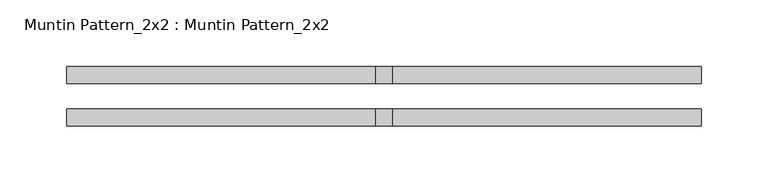
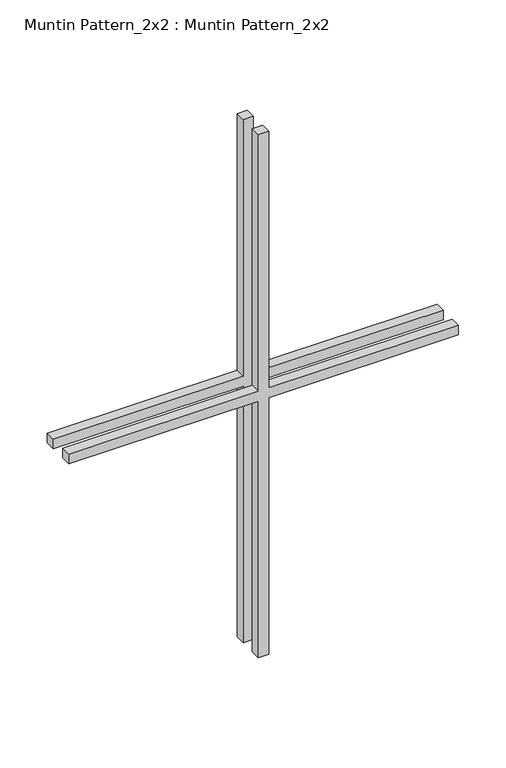
"""IFC4 building model written with IfcOpenShell, lengths in millimetres: proxy geometry, Muntin Pattern_2x2 : Muntin Pattern_2x2."""

from ifc_helpers import new_model, si_unit, frame, origin, place, context, project, spatial, polyline, outline, extrude, source, transform, mapped, element, save


def muntin_pattern_2x2_muntin_pattern_2x2_c58f38d7(model_context):
    return source(origin(), model_context, "Body", "SweptSolid", [
        extrude(outline(polyline([(342.9, -6.35), (342.9, -237.0666667), (330.2, -237.0666667), (330.2, -6.35), (0.0, -6.35), (0.0, 6.35), (330.2, 6.35), (330.2, 237.0666667), (342.9, 237.0666667), (342.9, 6.35), (673.1, 6.35), (673.1, -6.35), (342.9, -6.35)])), frame((0.0, -22.225, 0.0), z_axis=(0.0, 1.0, 0.0), x_axis=(0.0, 0.0, 1.0)), (0.0, 0.0, 1.0), 12.7),
        extrude(outline(polyline([(342.9, -6.35), (342.9, -237.0666667), (330.2, -237.0666667), (330.2, -6.35), (0.0, -6.35), (0.0, 6.35), (330.2, 6.35), (330.2, 237.0666667), (342.9, 237.0666667), (342.9, 6.35), (673.1, 6.35), (673.1, -6.35), (342.9, -6.35)])), frame((0.0, 9.525, 0.0), z_axis=(0.0, 1.0, 0.0), x_axis=(0.0, 0.0, 1.0)), (0.0, 0.0, 1.0), 12.7),
    ])


if __name__ == "__main__":
    model = new_model("IFC4")
    model_context = context("Model", 3, world=origin())
    ifc_project = project(units=[si_unit("LENGTHUNIT", "METRE", prefix="MILLI")], contexts=[model_context])
    site = spatial("IfcSite", under=ifc_project)
    building = spatial("IfcBuilding", under=site)
    placement = place(None, origin())
    muntin_pattern_2x2_muntin_pattern_2x2_shape = muntin_pattern_2x2_muntin_pattern_2x2_c58f38d7(model_context)
    element("IfcBuildingElementProxy", 1, Name="Muntin Pattern_2x2 : Muntin Pattern_2x2", ObjectType="Muntin Pattern_2x2 : Muntin Pattern_2x2", at=placement, inside=building, context=model_context, shape_type="MappedRepresentation", body=[
        mapped(muntin_pattern_2x2_muntin_pattern_2x2_shape, transform((0.0, 0.0, 0.0), x_axis=(1.0, 0.0, 0.0), y_axis=(0.0, 1.0, 0.0), z_axis=(0.0, 0.0, 1.0))),
    ])
    save(model, "model.ifc")

# Revit data of these elements
# Type "Muntin Pattern_2x2 : Muntin Pattern_2x2"
#   Width [instance default] = 4 ft
#   Thickness = 0.041667 ft
#   Height [instance default] = 4 ft
#   Distance = 0.0625 ft
#   Interior Material [instance default] = none
#   Exterior Material [instance default] = none
#   Default Elevation = 0
# Element 1 (IfcBuildingElementProxy, "Muntin Pattern_2x2 : Muntin Pattern_2x2")
#   Width = 1.555556 ft
#   Height = 2.208333 ft
#   Interior Material = Wood - Stained
#   Exterior Material = Clad - White
#   Materials on its faces: "Clad - White", "Wood - Stained"
# Materials
#   "Clad - White": class "Wood", colour RGB 242 242 238, transparency 0, Cost = 0
#   "Wood - Stained": class "Wood", colour RGB 224 178 126, transparency 0, Cost = 0
